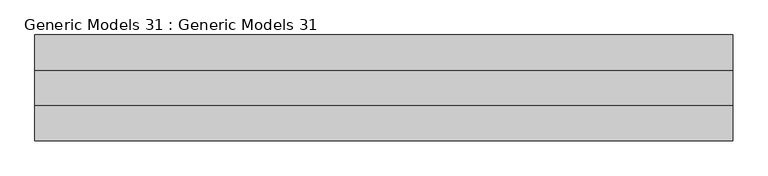
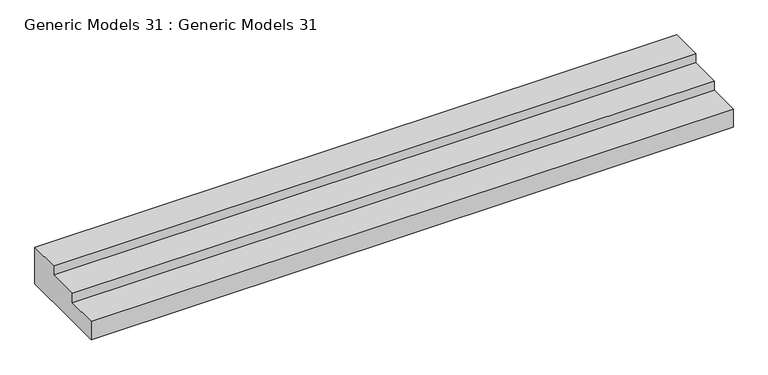
"""IFC4 building model written with IfcOpenShell, lengths in millimetres: proxy geometry, Generic Models 31 : Generic Models 31."""

from ifc_helpers import new_model, si_unit, frame, origin, place, context, project, spatial, polyline, outline, extrude, source, transform, mapped, element, save


def generic_models_31_generic_models_31_aad501af(model_context):
    return source(origin(), model_context, "Body", "SweptSolid", [
        extrude(outline(polyline([(-8147.9432518, 0.0), (-8624.1932518, 0.0), (-8909.9432518, 0.0), (-8909.9432518, 152.4), (-8655.9432518, 152.4), (-8655.9432518, 228.6), (-8401.9432518, 228.6), (-8401.9432518, 304.8), (-8147.9432518, 304.8), (-8147.9432518, 0.0)])), frame((-3134.5781265, 0.0, 0.0), z_axis=(1.0, 0.0, 0.0), x_axis=(0.0, 1.0, 0.0)), (0.0, 0.0, 1.0), 5030.4355479),
    ])


if __name__ == "__main__":
    model = new_model("IFC4")
    model_context = context("Model", 3, world=origin())
    ifc_project = project(units=[si_unit("LENGTHUNIT", "METRE", prefix="MILLI")], contexts=[model_context])
    site = spatial("IfcSite", under=ifc_project)
    building = spatial("IfcBuilding", under=site)
    placement = place(None, origin())
    generic_models_31_generic_models_31_shape = generic_models_31_generic_models_31_aad501af(model_context)
    element("IfcBuildingElementProxy", 1, Name="Generic Models 31 : Generic Models 31", ObjectType="Generic Models 31 : Generic Models 31", at=placement, inside=building, context=model_context, shape_type="MappedRepresentation", body=[
        mapped(generic_models_31_generic_models_31_shape, transform((0.0, 0.0, 0.0), x_axis=(1.0, 0.0, 0.0), y_axis=(0.0, 1.0, 0.0), z_axis=(0.0, 0.0, 1.0))),
    ])
    save(model, "model.ifc")
